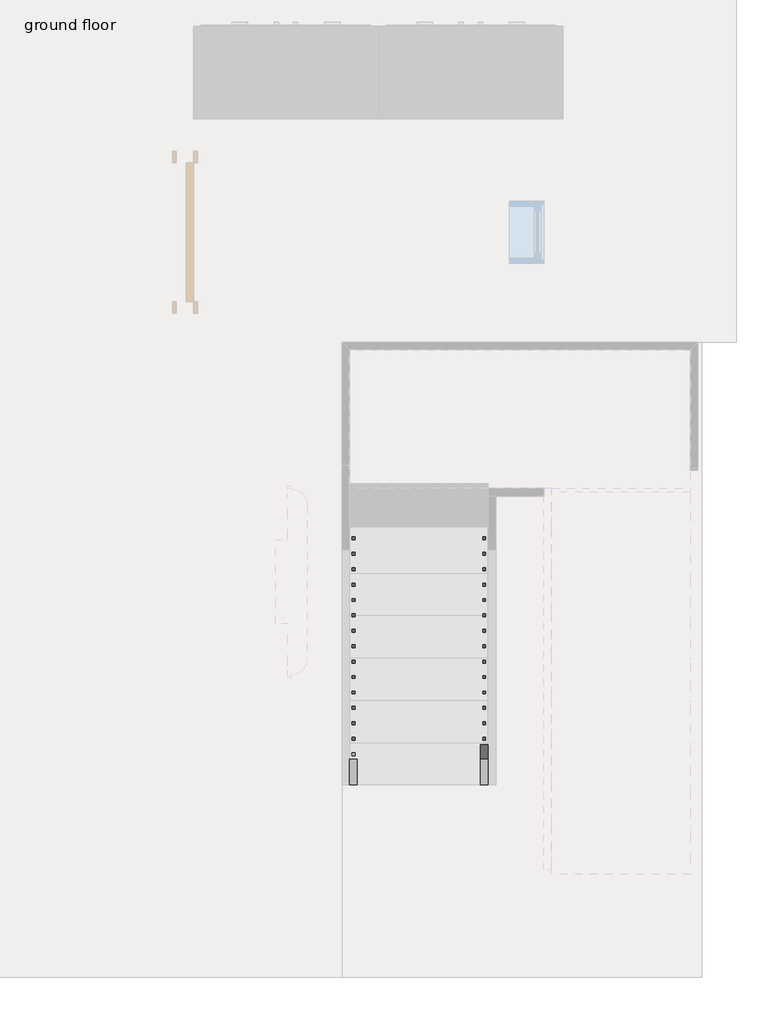
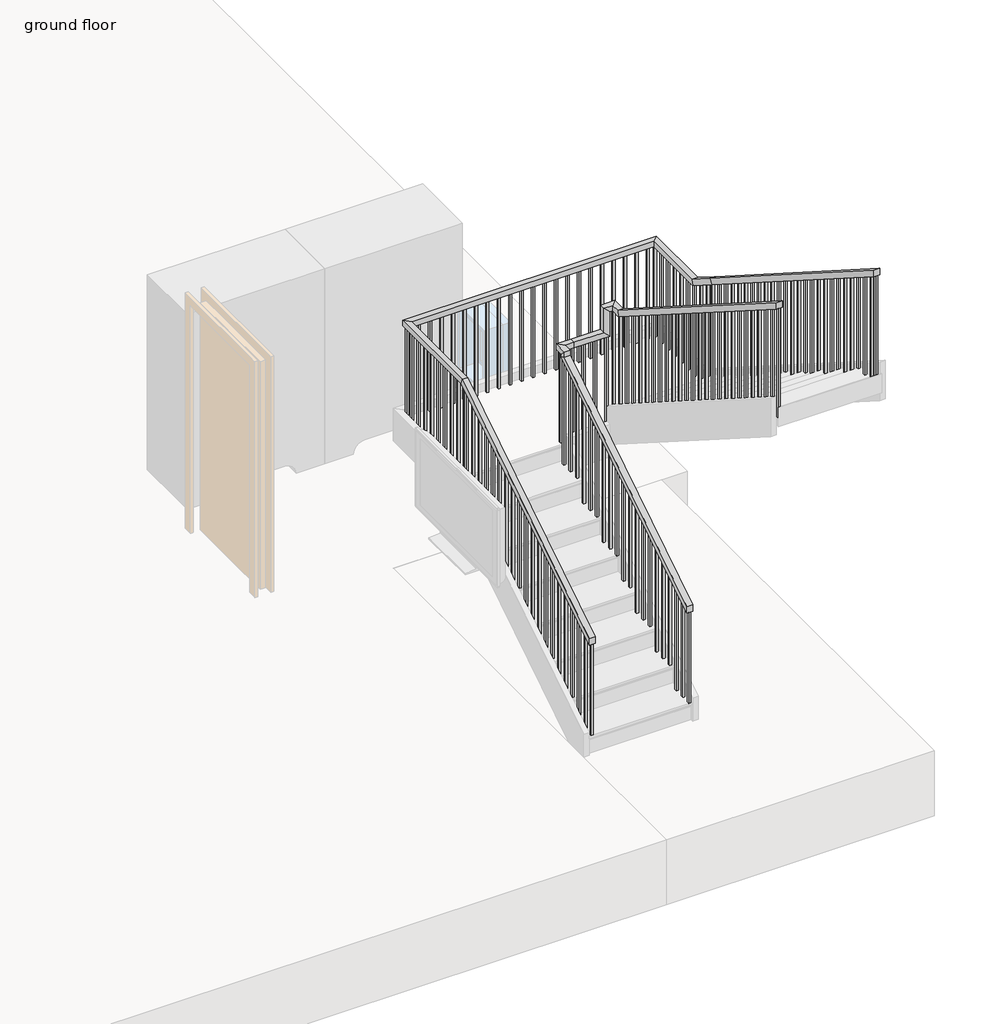
# One storey, part 2 of 3: 2 railings.
"""IFC4 building model written with IfcOpenShell, lengths in millimetres."""

from ifc_helpers import new_model, si_unit, frame, origin, place, context, project, spatial, polyline, outline, extrude, faceted_brep, element, save

model = new_model("IFC4")

# Units and contexts
model_context = context("Model", 3, world=origin())
ifc_project = project(units=[si_unit("LENGTHUNIT", "METRE", prefix="MILLI")], contexts=[model_context])

# Site, building, storey
site = spatial("IfcSite", under=ifc_project)
building = spatial("IfcBuilding", under=site)
storey = spatial("IfcBuildingStorey", under=building, Name="ground floor", Elevation=609.6)

# Railings
placement = place(None, origin())
element("IfcRailing", 1, ObjectType="Handrail - Rectangular", at=placement, inside=storey, context=model_context, shape_type="SolidModel", body=[
    faceted_brep([(995.5501403, 157.6257925, 1701.8), (995.5501403, 157.6257925, 1641.586276), (1046.3501403, 157.6257925, 1641.586276), (1046.3501403, 157.6257925, 1701.8), (995.5501403, 2037.2257925, 2897.9090909), (995.5501403, 2088.0257925, 2870.0226396), (1046.3501403, 2088.0257925, 2870.0226396), (1046.3501403, 2037.2257925, 2897.9090909), (995.5501403, 2037.2257925, 2946.4), (995.5501403, 2088.0257925, 2895.6), (1046.3501403, 2088.0257925, 2895.6), (1046.3501403, 2037.2257925, 2946.4), (995.5501403, 2164.2257925, 2946.4), (995.5501403, 2164.2257925, 2895.6), (1046.3501403, 2113.4257925, 2895.6), (1046.3501403, 2113.4257925, 2946.4), (1122.5501403, 2164.2257925, 2946.4), (1122.5501403, 2164.2257925, 2895.6), (1122.5501403, 2113.4257925, 2895.6), (1122.5501403, 2113.4257925, 2946.4), (1389.2501403, 2164.2257925, 2946.4), (1440.0501403, 2164.2257925, 2895.6), (1440.0501403, 2113.4257925, 2895.6), (1389.2501403, 2113.4257925, 2946.4), (1389.2501403, 2164.2257925, 3172.6909091), (1440.0501403, 2164.2257925, 3121.8909091), (1440.0501403, 2113.4257925, 3121.8909091), (1389.2501403, 2113.4257925, 3172.6909091), (1516.2501403, 2164.2257925, 3172.6909091), (1516.2501403, 2164.2257925, 3121.8909091), (1465.4501403, 2113.4257925, 3121.8909091), (1465.4501403, 2113.4257925, 3172.6909091), (1516.2501403, 2037.2257925, 3172.6909091), (1516.2501403, 2022.4327976, 3121.8909091), (1465.4501403, 2022.4327976, 3121.8909091), (1465.4501403, 2037.2257925, 3172.6909091), (1516.2501403, -401.1742075, 4724.4), (1465.4501403, -401.1742075, 4724.4), (1465.4501403, -401.1742075, 4664.186276), (1516.2501403, -401.1742075, 4664.186276)], [[[0, 1, 2, 3]], [[1, 0, 4, 5]], [[2, 1, 5, 6]], [[3, 2, 6, 7]], [[0, 3, 7, 4]], [[5, 4, 8, 9]], [[6, 5, 9, 10]], [[7, 6, 10, 11]], [[4, 7, 11, 8]], [[9, 8, 12, 13]], [[10, 9, 13, 14]], [[11, 10, 14, 15]], [[8, 11, 15, 12]], [[13, 12, 16, 17]], [[14, 13, 17, 18]], [[15, 14, 18, 19]], [[12, 15, 19, 16]], [[17, 16, 20, 21]], [[18, 17, 21, 22]], [[19, 18, 22, 23]], [[16, 19, 23, 20]], [[21, 20, 24, 25]], [[22, 21, 25, 26]], [[23, 22, 26, 27]], [[20, 23, 27, 24]], [[25, 24, 28, 29]], [[26, 25, 29, 30]], [[27, 26, 30, 31]], [[24, 27, 31, 28]], [[29, 28, 32, 33]], [[30, 29, 33, 34]], [[31, 30, 34, 35]], [[28, 31, 35, 32]], [[36, 37, 38, 39]], [[33, 32, 36, 39]], [[34, 33, 39, 38]], [[35, 34, 38, 37]], [[32, 35, 37, 36]]]),
    extrude(outline(polyline([(-309.0992075, 4605.5930941), (-290.0492075, 4593.4703669), (-290.0492075, 3632.2), (-309.0992075, 3632.2), (-309.0992075, 4605.5930941)])), frame((1481.3251403, 0.0, 0.0), z_axis=(1.0, 0.0, 0.0), x_axis=(0.0, 1.0, 0.0)), (0.0, 0.0, 1.0), 19.05),
    extrude(outline(polyline([(-207.4992075, 4540.9385487), (-188.4492075, 4528.8158214), (-188.4492075, 3632.2), (-207.4992075, 3632.2), (-207.4992075, 4540.9385487)])), frame((1481.3251403, 0.0, 0.0), z_axis=(1.0, 0.0, 0.0), x_axis=(0.0, 1.0, 0.0)), (0.0, 0.0, 1.0), 19.05),
    extrude(outline(polyline([(-105.8992075, 4476.2840032), (-86.8492075, 4464.161276), (-86.8492075, 3454.4), (-105.8992075, 3454.4), (-105.8992075, 4476.2840032)])), frame((1481.3251403, 0.0, 0.0), z_axis=(1.0, 0.0, 0.0), x_axis=(0.0, 1.0, 0.0)), (0.0, 0.0, 1.0), 19.05),
    extrude(outline(polyline([(-4.2992075, 4411.6294578), (14.7507925, 4399.5067305), (14.7507925, 3454.4), (-4.2992075, 3454.4), (-4.2992075, 4411.6294578)])), frame((1481.3251403, 0.0, 0.0), z_axis=(1.0, 0.0, 0.0), x_axis=(0.0, 1.0, 0.0)), (0.0, 0.0, 1.0), 19.05),
    extrude(outline(polyline([(97.3007925, 4346.9749123), (116.3507925, 4334.8521851), (116.3507925, 3454.4), (97.3007925, 3454.4), (97.3007925, 4346.9749123)])), frame((1481.3251403, 0.0, 0.0), z_axis=(1.0, 0.0, 0.0), x_axis=(0.0, 1.0, 0.0)), (0.0, 0.0, 1.0), 19.05),
    extrude(outline(polyline([(198.9007925, 4282.3203669), (217.9507925, 4270.1976396), (217.9507925, 3276.6), (198.9007925, 3276.6), (198.9007925, 4282.3203669)])), frame((1481.3251403, 0.0, 0.0), z_axis=(1.0, 0.0, 0.0), x_axis=(0.0, 1.0, 0.0)), (0.0, 0.0, 1.0), 19.05),
    extrude(outline(polyline([(300.5007925, 4217.6658214), (319.5507925, 4205.5430941), (319.5507925, 3276.6), (300.5007925, 3276.6), (300.5007925, 4217.6658214)])), frame((1481.3251403, 0.0, 0.0), z_axis=(1.0, 0.0, 0.0), x_axis=(0.0, 1.0, 0.0)), (0.0, 0.0, 1.0), 19.05),
    extrude(outline(polyline([(402.1007925, 4153.011276), (421.1507925, 4140.8885487), (421.1507925, 3276.6), (402.1007925, 3276.6), (402.1007925, 4153.011276)])), frame((1481.3251403, 0.0, 0.0), z_axis=(1.0, 0.0, 0.0), x_axis=(0.0, 1.0, 0.0)), (0.0, 0.0, 1.0), 19.05),
    extrude(outline(polyline([(503.7007925, 4088.3567305), (522.7507925, 4076.2340032), (522.7507925, 3098.8), (503.7007925, 3098.8), (503.7007925, 4088.3567305)])), frame((1481.3251403, 0.0, 0.0), z_axis=(1.0, 0.0, 0.0), x_axis=(0.0, 1.0, 0.0)), (0.0, 0.0, 1.0), 19.05),
    extrude(outline(polyline([(605.3007925, 4023.7021851), (624.3507925, 4011.5794578), (624.3507925, 3098.8), (605.3007925, 3098.8), (605.3007925, 4023.7021851)])), frame((1481.3251403, 0.0, 0.0), z_axis=(1.0, 0.0, 0.0), x_axis=(0.0, 1.0, 0.0)), (0.0, 0.0, 1.0), 19.05),
    extrude(outline(polyline([(706.9007925, 3959.0476396), (725.9507925, 3946.9249123), (725.9507925, 3098.8), (706.9007925, 3098.8), (706.9007925, 3959.0476396)])), frame((1481.3251403, 0.0, 0.0), z_axis=(1.0, 0.0, 0.0), x_axis=(0.0, 1.0, 0.0)), (0.0, 0.0, 1.0), 19.05),
    extrude(outline(polyline([(808.5007925, 3894.3930941), (827.5507925, 3882.2703669), (827.5507925, 2921.0), (808.5007925, 2921.0), (808.5007925, 3894.3930941)])), frame((1481.3251403, 0.0, 0.0), z_axis=(1.0, 0.0, 0.0), x_axis=(0.0, 1.0, 0.0)), (0.0, 0.0, 1.0), 19.05),
    extrude(outline(polyline([(910.1007925, 3829.7385487), (929.1507925, 3817.6158214), (929.1507925, 2921.0), (910.1007925, 2921.0), (910.1007925, 3829.7385487)])), frame((1481.3251403, 0.0, 0.0), z_axis=(1.0, 0.0, 0.0), x_axis=(0.0, 1.0, 0.0)), (0.0, 0.0, 1.0), 19.05),
    extrude(outline(polyline([(1011.7007925, 3765.0840032), (1030.7507925, 3752.961276), (1030.7507925, 2743.2), (1011.7007925, 2743.2), (1011.7007925, 3765.0840032)])), frame((1481.3251403, 0.0, 0.0), z_axis=(1.0, 0.0, 0.0), x_axis=(0.0, 1.0, 0.0)), (0.0, 0.0, 1.0), 19.05),
    extrude(outline(polyline([(1113.3007925, 3700.4294578), (1132.3507925, 3688.3067305), (1132.3507925, 2743.2), (1113.3007925, 2743.2), (1113.3007925, 3700.4294578)])), frame((1481.3251403, 0.0, 0.0), z_axis=(1.0, 0.0, 0.0), x_axis=(0.0, 1.0, 0.0)), (0.0, 0.0, 1.0), 19.05),
    extrude(outline(polyline([(1214.9007925, 3635.7749123), (1233.9507925, 3623.6521851), (1233.9507925, 2743.2), (1214.9007925, 2743.2), (1214.9007925, 3635.7749123)])), frame((1481.3251403, 0.0, 0.0), z_axis=(1.0, 0.0, 0.0), x_axis=(0.0, 1.0, 0.0)), (0.0, 0.0, 1.0), 19.05),
    extrude(outline(polyline([(1316.5007925, 3571.1203669), (1335.5507925, 3558.9976396), (1335.5507925, 2565.4), (1316.5007925, 2565.4), (1316.5007925, 3571.1203669)])), frame((1481.3251403, 0.0, 0.0), z_axis=(1.0, 0.0, 0.0), x_axis=(0.0, 1.0, 0.0)), (0.0, 0.0, 1.0), 19.05),
    extrude(outline(polyline([(1418.1007925, 3506.4658214), (1437.1507925, 3494.3430941), (1437.1507925, 2565.4), (1418.1007925, 2565.4), (1418.1007925, 3506.4658214)])), frame((1481.3251403, 0.0, 0.0), z_axis=(1.0, 0.0, 0.0), x_axis=(0.0, 1.0, 0.0)), (0.0, 0.0, 1.0), 19.05),
    extrude(outline(polyline([(1519.7007925, 3441.811276), (1538.7507925, 3429.6885487), (1538.7507925, 2565.4), (1519.7007925, 2565.4), (1519.7007925, 3441.811276)])), frame((1481.3251403, 0.0, 0.0), z_axis=(1.0, 0.0, 0.0), x_axis=(0.0, 1.0, 0.0)), (0.0, 0.0, 1.0), 19.05),
    extrude(outline(polyline([(1621.3007925, 3377.1567305), (1640.3507925, 3365.0340032), (1640.3507925, 2387.6), (1621.3007925, 2387.6), (1621.3007925, 3377.1567305)])), frame((1481.3251403, 0.0, 0.0), z_axis=(1.0, 0.0, 0.0), x_axis=(0.0, 1.0, 0.0)), (0.0, 0.0, 1.0), 19.05),
    extrude(outline(polyline([(1722.9007925, 3312.5021851), (1741.9507925, 3300.3794578), (1741.9507925, 2387.6), (1722.9007925, 2387.6), (1722.9007925, 3312.5021851)])), frame((1481.3251403, 0.0, 0.0), z_axis=(1.0, 0.0, 0.0), x_axis=(0.0, 1.0, 0.0)), (0.0, 0.0, 1.0), 19.05),
    extrude(outline(polyline([(1824.5007925, 3247.8476396), (1843.5507925, 3235.7249123), (1843.5507925, 2387.6), (1824.5007925, 2387.6), (1824.5007925, 3247.8476396)])), frame((1481.3251403, 0.0, 0.0), z_axis=(1.0, 0.0, 0.0), x_axis=(0.0, 1.0, 0.0)), (0.0, 0.0, 1.0), 19.05),
    extrude(outline(polyline([(1926.1007925, 3183.1930941), (1945.1507925, 3171.0703669), (1945.1507925, 2209.8), (1926.1007925, 2209.8), (1926.1007925, 3183.1930941)])), frame((1481.3251403, 0.0, 0.0), z_axis=(1.0, 0.0, 0.0), x_axis=(0.0, 1.0, 0.0)), (0.0, 0.0, 1.0), 19.05),
    extrude(outline(polyline([(2027.7007925, 3118.5385487), (2046.7507925, 3106.4158214), (2046.7507925, 2209.8), (2027.7007925, 2209.8), (2027.7007925, 3118.5385487)])), frame((1481.3251403, 0.0, 0.0), z_axis=(1.0, 0.0, 0.0), x_axis=(0.0, 1.0, 0.0)), (0.0, 0.0, 1.0), 19.05),
    extrude(outline(polyline([(1417.8251403, 2129.3007925), (1417.8251403, 2148.3507925), (1436.8751403, 2148.3507925), (1436.8751403, 2129.3007925), (1417.8251403, 2129.3007925)])), frame((0.0, 0.0, 2032.0), z_axis=(0.0, 0.0, 1.0), x_axis=(1.0, 0.0, 0.0)), (0.0, 0.0, 1.0), 1089.8909091),
    extrude(outline(polyline([(1316.2251403, 2129.3007925), (1316.2251403, 2148.3507925), (1335.2751403, 2148.3507925), (1335.2751403, 2129.3007925), (1316.2251403, 2129.3007925)])), frame((0.0, 0.0, 2032.0), z_axis=(0.0, 0.0, 1.0), x_axis=(1.0, 0.0, 0.0)), (0.0, 0.0, 1.0), 863.6),
    extrude(outline(polyline([(1214.6251403, 2129.3007925), (1214.6251403, 2148.3507925), (1233.6751403, 2148.3507925), (1233.6751403, 2129.3007925), (1214.6251403, 2129.3007925)])), frame((0.0, 0.0, 2032.0), z_axis=(0.0, 0.0, 1.0), x_axis=(1.0, 0.0, 0.0)), (0.0, 0.0, 1.0), 863.6),
    extrude(outline(polyline([(1113.0251403, 2129.3007925), (1113.0251403, 2148.3507925), (1132.0751403, 2148.3507925), (1132.0751403, 2129.3007925), (1113.0251403, 2129.3007925)])), frame((0.0, 0.0, 2032.0), z_axis=(0.0, 0.0, 1.0), x_axis=(1.0, 0.0, 0.0)), (0.0, 0.0, 1.0), 863.6),
    extrude(outline(polyline([(1030.4751403, 2078.5007925), (1011.4251403, 2078.5007925), (1011.4251403, 2097.5507925), (1030.4751403, 2097.5507925), (1030.4751403, 2078.5007925)])), frame((0.0, 0.0, 1854.2), z_axis=(0.0, 0.0, 1.0), x_axis=(1.0, 0.0, 0.0)), (0.0, 0.0, 1.0), 1041.4),
    extrude(outline(polyline([(1976.9007925, 2799.3067305), (1995.9507925, 2811.4294578), (1995.9507925, 1854.2), (1976.9007925, 1854.2), (1976.9007925, 2799.3067305)])), frame((1011.4251403, 0.0, 0.0), z_axis=(1.0, 0.0, 0.0), x_axis=(0.0, 1.0, 0.0)), (0.0, 0.0, 1.0), 19.05),
    extrude(outline(polyline([(1875.3007925, 2734.6521851), (1894.3507925, 2746.7749123), (1894.3507925, 1854.2), (1875.3007925, 1854.2), (1875.3007925, 2734.6521851)])), frame((1011.4251403, 0.0, 0.0), z_axis=(1.0, 0.0, 0.0), x_axis=(0.0, 1.0, 0.0)), (0.0, 0.0, 1.0), 19.05),
    extrude(outline(polyline([(1773.7007925, 2669.9976396), (1792.7507925, 2682.1203669), (1792.7507925, 1676.4), (1773.7007925, 1676.4), (1773.7007925, 2669.9976396)])), frame((1011.4251403, 0.0, 0.0), z_axis=(1.0, 0.0, 0.0), x_axis=(0.0, 1.0, 0.0)), (0.0, 0.0, 1.0), 19.05),
    extrude(outline(polyline([(1672.1007925, 2605.3430941), (1691.1507925, 2617.4658214), (1691.1507925, 1676.4), (1672.1007925, 1676.4), (1672.1007925, 2605.3430941)])), frame((1011.4251403, 0.0, 0.0), z_axis=(1.0, 0.0, 0.0), x_axis=(0.0, 1.0, 0.0)), (0.0, 0.0, 1.0), 19.05),
    extrude(outline(polyline([(1570.5007925, 2540.6885487), (1589.5507925, 2552.811276), (1589.5507925, 1676.4), (1570.5007925, 1676.4), (1570.5007925, 2540.6885487)])), frame((1011.4251403, 0.0, 0.0), z_axis=(1.0, 0.0, 0.0), x_axis=(0.0, 1.0, 0.0)), (0.0, 0.0, 1.0), 19.05),
    extrude(outline(polyline([(1468.9007925, 2476.0340032), (1487.9507925, 2488.1567305), (1487.9507925, 1498.6), (1468.9007925, 1498.6), (1468.9007925, 2476.0340032)])), frame((1011.4251403, 0.0, 0.0), z_axis=(1.0, 0.0, 0.0), x_axis=(0.0, 1.0, 0.0)), (0.0, 0.0, 1.0), 19.05),
    extrude(outline(polyline([(1367.3007925, 2411.3794578), (1386.3507925, 2423.5021851), (1386.3507925, 1498.6), (1367.3007925, 1498.6), (1367.3007925, 2411.3794578)])), frame((1011.4251403, 0.0, 0.0), z_axis=(1.0, 0.0, 0.0), x_axis=(0.0, 1.0, 0.0)), (0.0, 0.0, 1.0), 19.05),
    extrude(outline(polyline([(1265.7007925, 2346.7249123), (1284.7507925, 2358.8476396), (1284.7507925, 1498.6), (1265.7007925, 1498.6), (1265.7007925, 2346.7249123)])), frame((1011.4251403, 0.0, 0.0), z_axis=(1.0, 0.0, 0.0), x_axis=(0.0, 1.0, 0.0)), (0.0, 0.0, 1.0), 19.05),
    extrude(outline(polyline([(1164.1007925, 2282.0703669), (1183.1507925, 2294.1930941), (1183.1507925, 1320.8), (1164.1007925, 1320.8), (1164.1007925, 2282.0703669)])), frame((1011.4251403, 0.0, 0.0), z_axis=(1.0, 0.0, 0.0), x_axis=(0.0, 1.0, 0.0)), (0.0, 0.0, 1.0), 19.05),
    extrude(outline(polyline([(1062.5007925, 2217.4158214), (1081.5507925, 2229.5385487), (1081.5507925, 1320.8), (1062.5007925, 1320.8), (1062.5007925, 2217.4158214)])), frame((1011.4251403, 0.0, 0.0), z_axis=(1.0, 0.0, 0.0), x_axis=(0.0, 1.0, 0.0)), (0.0, 0.0, 1.0), 19.05),
    extrude(outline(polyline([(960.9007925, 2152.761276), (979.9507925, 2164.8840032), (979.9507925, 1143.0), (960.9007925, 1143.0), (960.9007925, 2152.761276)])), frame((1011.4251403, 0.0, 0.0), z_axis=(1.0, 0.0, 0.0), x_axis=(0.0, 1.0, 0.0)), (0.0, 0.0, 1.0), 19.05),
    extrude(outline(polyline([(859.3007925, 2088.1067305), (878.3507925, 2100.2294578), (878.3507925, 1143.0), (859.3007925, 1143.0), (859.3007925, 2088.1067305)])), frame((1011.4251403, 0.0, 0.0), z_axis=(1.0, 0.0, 0.0), x_axis=(0.0, 1.0, 0.0)), (0.0, 0.0, 1.0), 19.05),
    extrude(outline(polyline([(757.7007925, 2023.4521851), (776.7507925, 2035.5749123), (776.7507925, 1143.0), (757.7007925, 1143.0), (757.7007925, 2023.4521851)])), frame((1011.4251403, 0.0, 0.0), z_axis=(1.0, 0.0, 0.0), x_axis=(0.0, 1.0, 0.0)), (0.0, 0.0, 1.0), 19.05),
    extrude(outline(polyline([(656.1007925, 1958.7976396), (675.1507925, 1970.9203669), (675.1507925, 965.2), (656.1007925, 965.2), (656.1007925, 1958.7976396)])), frame((1011.4251403, 0.0, 0.0), z_axis=(1.0, 0.0, 0.0), x_axis=(0.0, 1.0, 0.0)), (0.0, 0.0, 1.0), 19.05),
    extrude(outline(polyline([(554.5007925, 1894.1430941), (573.5507925, 1906.2658214), (573.5507925, 965.2), (554.5007925, 965.2), (554.5007925, 1894.1430941)])), frame((1011.4251403, 0.0, 0.0), z_axis=(1.0, 0.0, 0.0), x_axis=(0.0, 1.0, 0.0)), (0.0, 0.0, 1.0), 19.05),
    extrude(outline(polyline([(452.9007925, 1829.4885487), (471.9507925, 1841.611276), (471.9507925, 965.2), (452.9007925, 965.2), (452.9007925, 1829.4885487)])), frame((1011.4251403, 0.0, 0.0), z_axis=(1.0, 0.0, 0.0), x_axis=(0.0, 1.0, 0.0)), (0.0, 0.0, 1.0), 19.05),
    extrude(outline(polyline([(351.3007925, 1764.8340032), (370.3507925, 1776.9567305), (370.3507925, 787.4), (351.3007925, 787.4), (351.3007925, 1764.8340032)])), frame((1011.4251403, 0.0, 0.0), z_axis=(1.0, 0.0, 0.0), x_axis=(0.0, 1.0, 0.0)), (0.0, 0.0, 1.0), 19.05),
    extrude(outline(polyline([(249.7007925, 1700.1794578), (268.7507925, 1712.3021851), (268.7507925, 787.4), (249.7007925, 787.4), (249.7007925, 1700.1794578)])), frame((1011.4251403, 0.0, 0.0), z_axis=(1.0, 0.0, 0.0), x_axis=(0.0, 1.0, 0.0)), (0.0, 0.0, 1.0), 19.05),
    extrude(outline(polyline([(1481.3251403, 2129.3007925), (1481.3251403, 2148.3507925), (1500.3751403, 2148.3507925), (1500.3751403, 2129.3007925), (1481.3251403, 2129.3007925)])), frame((0.0, 0.0, 2032.0), z_axis=(0.0, 0.0, 1.0), x_axis=(1.0, 0.0, 0.0)), (0.0, 0.0, 1.0), 1089.8909091),
    extrude(outline(polyline([(1030.4751403, 2129.3007925), (1011.4251403, 2129.3007925), (1011.4251403, 2148.3507925), (1030.4751403, 2148.3507925), (1030.4751403, 2129.3007925)])), frame((0.0, 0.0, 2032.0), z_axis=(0.0, 0.0, 1.0), x_axis=(1.0, 0.0, 0.0)), (0.0, 0.0, 1.0), 863.6),
    extrude(outline(polyline([(-401.1742075, 4664.186276), (-382.1242075, 4652.0635487), (-382.1242075, 3632.2), (-401.1742075, 3632.2), (-401.1742075, 4664.186276)])), frame((1481.3251403, 0.0, 0.0), z_axis=(1.0, 0.0, 0.0), x_axis=(0.0, 1.0, 0.0)), (0.0, 0.0, 1.0), 19.05),
    extrude(outline(polyline([(157.6257925, 1641.586276), (176.6757925, 1653.7090032), (176.6757925, 787.4), (157.6257925, 787.4), (157.6257925, 1641.586276)])), frame((1011.4251403, 0.0, 0.0), z_axis=(1.0, 0.0, 0.0), x_axis=(0.0, 1.0, 0.0)), (0.0, 0.0, 1.0), 19.05),
])
element("IfcRailing", 2, ObjectType="Handrail - Rectangular", at=placement, inside=storey, context=model_context, shape_type="SolidModel", body=[
    faceted_brep([(131.9501403, 157.6257925, 1701.8), (131.9501403, 157.6257925, 1641.586276), (182.7501403, 157.6257925, 1641.586276), (182.7501403, 157.6257925, 1701.8), (131.9501403, 2113.4257925, 2946.4), (131.9501403, 2128.2187874, 2895.6), (182.7501403, 2128.2187874, 2895.6), (182.7501403, 2113.4257925, 2946.4), (131.9501403, 3027.8257925, 2946.4), (131.9501403, 3027.8257925, 2895.6), (182.7501403, 2977.0257925, 2895.6), (182.7501403, 2977.0257925, 2946.4), (2379.8501403, 3027.8257925, 2946.4), (2379.8501403, 3027.8257925, 2895.6), (2329.0501403, 2977.0257925, 2895.6), (2329.0501403, 2977.0257925, 2946.4), (2379.8501403, 2392.8257925, 2946.4), (2379.8501403, 2378.0327976, 2895.6), (2329.0501403, 2378.0327976, 2895.6), (2329.0501403, 2392.8257925, 2946.4), (2379.8501403, 2113.4257925, 3124.2), (2379.8501403, 2086.1525175, 3081.3419964), (2329.0501403, 2086.1525175, 3081.3419964), (2329.0501403, 2113.4257925, 3124.2), (2379.8501403, -401.1742075, 4724.4), (2329.0501403, -401.1742075, 4724.4), (2329.0501403, -401.1742075, 4664.186276), (2379.8501403, -401.1742075, 4664.186276)], [[[0, 1, 2, 3]], [[1, 0, 4, 5]], [[2, 1, 5, 6]], [[3, 2, 6, 7]], [[0, 3, 7, 4]], [[5, 4, 8, 9]], [[6, 5, 9, 10]], [[7, 6, 10, 11]], [[4, 7, 11, 8]], [[9, 8, 12, 13]], [[10, 9, 13, 14]], [[11, 10, 14, 15]], [[8, 11, 15, 12]], [[13, 12, 16, 17]], [[14, 13, 17, 18]], [[15, 14, 18, 19]], [[12, 15, 19, 16]], [[17, 16, 20, 21]], [[18, 17, 21, 22]], [[19, 18, 22, 23]], [[16, 19, 23, 20]], [[24, 25, 26, 27]], [[21, 20, 24, 27]], [[22, 21, 27, 26]], [[23, 22, 26, 25]], [[20, 23, 25, 24]]]),
    extrude(outline(polyline([(-315.4492075, 4609.6340032), (-315.4492075, 3632.2), (-334.4992075, 3632.2), (-334.4992075, 4621.7567305), (-315.4492075, 4609.6340032)])), frame((2344.9251403, 0.0, 0.0), z_axis=(1.0, 0.0, 0.0), x_axis=(0.0, 1.0, 0.0)), (0.0, 0.0, 1.0), 19.05),
    extrude(outline(polyline([(-213.8492075, 4544.9794578), (-213.8492075, 3632.2), (-232.8992075, 3632.2), (-232.8992075, 4557.1021851), (-213.8492075, 4544.9794578)])), frame((2344.9251403, 0.0, 0.0), z_axis=(1.0, 0.0, 0.0), x_axis=(0.0, 1.0, 0.0)), (0.0, 0.0, 1.0), 19.05),
    extrude(outline(polyline([(-112.2492075, 4480.3249123), (-112.2492075, 3632.2), (-131.2992075, 3632.2), (-131.2992075, 4492.4476396), (-112.2492075, 4480.3249123)])), frame((2344.9251403, 0.0, 0.0), z_axis=(1.0, 0.0, 0.0), x_axis=(0.0, 1.0, 0.0)), (0.0, 0.0, 1.0), 19.05),
    extrude(outline(polyline([(-10.6492075, 4415.6703669), (-10.6492075, 3454.4), (-29.6992075, 3454.4), (-29.6992075, 4427.7930941), (-10.6492075, 4415.6703669)])), frame((2344.9251403, 0.0, 0.0), z_axis=(1.0, 0.0, 0.0), x_axis=(0.0, 1.0, 0.0)), (0.0, 0.0, 1.0), 19.05),
    extrude(outline(polyline([(90.9507925, 4351.0158214), (90.9507925, 3454.4), (71.9007925, 3454.4), (71.9007925, 4363.1385487), (90.9507925, 4351.0158214)])), frame((2344.9251403, 0.0, 0.0), z_axis=(1.0, 0.0, 0.0), x_axis=(0.0, 1.0, 0.0)), (0.0, 0.0, 1.0), 19.05),
    extrude(outline(polyline([(192.5507925, 4286.361276), (192.5507925, 3276.6), (173.5007925, 3276.6), (173.5007925, 4298.4840032), (192.5507925, 4286.361276)])), frame((2344.9251403, 0.0, 0.0), z_axis=(1.0, 0.0, 0.0), x_axis=(0.0, 1.0, 0.0)), (0.0, 0.0, 1.0), 19.05),
    extrude(outline(polyline([(294.1507925, 4221.7067305), (294.1507925, 3276.6), (275.1007925, 3276.6), (275.1007925, 4233.8294578), (294.1507925, 4221.7067305)])), frame((2344.9251403, 0.0, 0.0), z_axis=(1.0, 0.0, 0.0), x_axis=(0.0, 1.0, 0.0)), (0.0, 0.0, 1.0), 19.05),
    extrude(outline(polyline([(395.7507925, 4157.0521851), (395.7507925, 3276.6), (376.7007925, 3276.6), (376.7007925, 4169.1749123), (395.7507925, 4157.0521851)])), frame((2344.9251403, 0.0, 0.0), z_axis=(1.0, 0.0, 0.0), x_axis=(0.0, 1.0, 0.0)), (0.0, 0.0, 1.0), 19.05),
    extrude(outline(polyline([(497.3507925, 4092.3976396), (497.3507925, 3098.8), (478.3007925, 3098.8), (478.3007925, 4104.5203669), (497.3507925, 4092.3976396)])), frame((2344.9251403, 0.0, 0.0), z_axis=(1.0, 0.0, 0.0), x_axis=(0.0, 1.0, 0.0)), (0.0, 0.0, 1.0), 19.05),
    extrude(outline(polyline([(598.9507925, 4027.7430941), (598.9507925, 3098.8), (579.9007925, 3098.8), (579.9007925, 4039.8658214), (598.9507925, 4027.7430941)])), frame((2344.9251403, 0.0, 0.0), z_axis=(1.0, 0.0, 0.0), x_axis=(0.0, 1.0, 0.0)), (0.0, 0.0, 1.0), 19.05),
    extrude(outline(polyline([(700.5507925, 3963.0885487), (700.5507925, 3098.8), (681.5007925, 3098.8), (681.5007925, 3975.211276), (700.5507925, 3963.0885487)])), frame((2344.9251403, 0.0, 0.0), z_axis=(1.0, 0.0, 0.0), x_axis=(0.0, 1.0, 0.0)), (0.0, 0.0, 1.0), 19.05),
    extrude(outline(polyline([(802.1507925, 3898.4340032), (802.1507925, 2921.0), (783.1007925, 2921.0), (783.1007925, 3910.5567305), (802.1507925, 3898.4340032)])), frame((2344.9251403, 0.0, 0.0), z_axis=(1.0, 0.0, 0.0), x_axis=(0.0, 1.0, 0.0)), (0.0, 0.0, 1.0), 19.05),
    extrude(outline(polyline([(903.7507925, 3833.7794578), (903.7507925, 2921.0), (884.7007925, 2921.0), (884.7007925, 3845.9021851), (903.7507925, 3833.7794578)])), frame((2344.9251403, 0.0, 0.0), z_axis=(1.0, 0.0, 0.0), x_axis=(0.0, 1.0, 0.0)), (0.0, 0.0, 1.0), 19.05),
    extrude(outline(polyline([(1005.3507925, 3769.1249123), (1005.3507925, 2921.0), (986.3007925, 2921.0), (986.3007925, 3781.2476396), (1005.3507925, 3769.1249123)])), frame((2344.9251403, 0.0, 0.0), z_axis=(1.0, 0.0, 0.0), x_axis=(0.0, 1.0, 0.0)), (0.0, 0.0, 1.0), 19.05),
    extrude(outline(polyline([(1106.9507925, 3704.4703669), (1106.9507925, 2743.2), (1087.9007925, 2743.2), (1087.9007925, 3716.5930941), (1106.9507925, 3704.4703669)])), frame((2344.9251403, 0.0, 0.0), z_axis=(1.0, 0.0, 0.0), x_axis=(0.0, 1.0, 0.0)), (0.0, 0.0, 1.0), 19.05),
    extrude(outline(polyline([(1208.5507925, 3639.8158214), (1208.5507925, 2743.2), (1189.5007925, 2743.2), (1189.5007925, 3651.9385487), (1208.5507925, 3639.8158214)])), frame((2344.9251403, 0.0, 0.0), z_axis=(1.0, 0.0, 0.0), x_axis=(0.0, 1.0, 0.0)), (0.0, 0.0, 1.0), 19.05),
    extrude(outline(polyline([(1310.1507925, 3575.161276), (1310.1507925, 2565.4), (1291.1007925, 2565.4), (1291.1007925, 3587.2840032), (1310.1507925, 3575.161276)])), frame((2344.9251403, 0.0, 0.0), z_axis=(1.0, 0.0, 0.0), x_axis=(0.0, 1.0, 0.0)), (0.0, 0.0, 1.0), 19.05),
    extrude(outline(polyline([(1411.7507925, 3510.5067305), (1411.7507925, 2565.4), (1392.7007925, 2565.4), (1392.7007925, 3522.6294578), (1411.7507925, 3510.5067305)])), frame((2344.9251403, 0.0, 0.0), z_axis=(1.0, 0.0, 0.0), x_axis=(0.0, 1.0, 0.0)), (0.0, 0.0, 1.0), 19.05),
    extrude(outline(polyline([(1513.3507925, 3445.8521851), (1513.3507925, 2565.4), (1494.3007925, 2565.4), (1494.3007925, 3457.9749123), (1513.3507925, 3445.8521851)])), frame((2344.9251403, 0.0, 0.0), z_axis=(1.0, 0.0, 0.0), x_axis=(0.0, 1.0, 0.0)), (0.0, 0.0, 1.0), 19.05),
    extrude(outline(polyline([(1614.9507925, 3381.1976396), (1614.9507925, 2387.6), (1595.9007925, 2387.6), (1595.9007925, 3393.3203669), (1614.9507925, 3381.1976396)])), frame((2344.9251403, 0.0, 0.0), z_axis=(1.0, 0.0, 0.0), x_axis=(0.0, 1.0, 0.0)), (0.0, 0.0, 1.0), 19.05),
    extrude(outline(polyline([(1716.5507925, 3316.5430941), (1716.5507925, 2387.6), (1697.5007925, 2387.6), (1697.5007925, 3328.6658214), (1716.5507925, 3316.5430941)])), frame((2344.9251403, 0.0, 0.0), z_axis=(1.0, 0.0, 0.0), x_axis=(0.0, 1.0, 0.0)), (0.0, 0.0, 1.0), 19.05),
    extrude(outline(polyline([(1818.1507925, 3251.8885487), (1818.1507925, 2387.6), (1799.1007925, 2387.6), (1799.1007925, 3264.011276), (1818.1507925, 3251.8885487)])), frame((2344.9251403, 0.0, 0.0), z_axis=(1.0, 0.0, 0.0), x_axis=(0.0, 1.0, 0.0)), (0.0, 0.0, 1.0), 19.05),
    extrude(outline(polyline([(1919.7507925, 3187.2340032), (1919.7507925, 2209.8), (1900.7007925, 2209.8), (1900.7007925, 3199.3567305), (1919.7507925, 3187.2340032)])), frame((2344.9251403, 0.0, 0.0), z_axis=(1.0, 0.0, 0.0), x_axis=(0.0, 1.0, 0.0)), (0.0, 0.0, 1.0), 19.05),
    extrude(outline(polyline([(2021.3507925, 3122.5794578), (2021.3507925, 2209.8), (2002.3007925, 2209.8), (2002.3007925, 3134.7021851), (2021.3507925, 3122.5794578)])), frame((2344.9251403, 0.0, 0.0), z_axis=(1.0, 0.0, 0.0), x_axis=(0.0, 1.0, 0.0)), (0.0, 0.0, 1.0), 19.05),
    extrude(outline(polyline([(2199.1507925, 3009.4340032), (2199.1507925, 2032.0), (2180.1007925, 2032.0), (2180.1007925, 3021.5567305), (2199.1507925, 3009.4340032)])), frame((2344.9251403, 0.0, 0.0), z_axis=(1.0, 0.0, 0.0), x_axis=(0.0, 1.0, 0.0)), (0.0, 0.0, 1.0), 19.05),
    extrude(outline(polyline([(2300.7507925, 2944.7794578), (2300.7507925, 2032.0), (2281.7007925, 2032.0), (2281.7007925, 2956.9021851), (2300.7507925, 2944.7794578)])), frame((2344.9251403, 0.0, 0.0), z_axis=(1.0, 0.0, 0.0), x_axis=(0.0, 1.0, 0.0)), (0.0, 0.0, 1.0), 19.05),
    extrude(outline(polyline([(2363.9751403, 2402.3507925), (2363.9751403, 2383.3007925), (2344.9251403, 2383.3007925), (2344.9251403, 2402.3507925), (2363.9751403, 2402.3507925)])), frame((0.0, 0.0, 2032.0), z_axis=(0.0, 0.0, 1.0), x_axis=(1.0, 0.0, 0.0)), (0.0, 0.0, 1.0), 863.6),
    extrude(outline(polyline([(2363.9751403, 2503.9507925), (2363.9751403, 2484.9007925), (2344.9251403, 2484.9007925), (2344.9251403, 2503.9507925), (2363.9751403, 2503.9507925)])), frame((0.0, 0.0, 2032.0), z_axis=(0.0, 0.0, 1.0), x_axis=(1.0, 0.0, 0.0)), (0.0, 0.0, 1.0), 863.6),
    extrude(outline(polyline([(2363.9751403, 2605.5507925), (2363.9751403, 2586.5007925), (2344.9251403, 2586.5007925), (2344.9251403, 2605.5507925), (2363.9751403, 2605.5507925)])), frame((0.0, 0.0, 2032.0), z_axis=(0.0, 0.0, 1.0), x_axis=(1.0, 0.0, 0.0)), (0.0, 0.0, 1.0), 863.6),
    extrude(outline(polyline([(2363.9751403, 2707.1507925), (2363.9751403, 2688.1007925), (2344.9251403, 2688.1007925), (2344.9251403, 2707.1507925), (2363.9751403, 2707.1507925)])), frame((0.0, 0.0, 2032.0), z_axis=(0.0, 0.0, 1.0), x_axis=(1.0, 0.0, 0.0)), (0.0, 0.0, 1.0), 863.6),
    extrude(outline(polyline([(2363.9751403, 2808.7507925), (2363.9751403, 2789.7007925), (2344.9251403, 2789.7007925), (2344.9251403, 2808.7507925), (2363.9751403, 2808.7507925)])), frame((0.0, 0.0, 2032.0), z_axis=(0.0, 0.0, 1.0), x_axis=(1.0, 0.0, 0.0)), (0.0, 0.0, 1.0), 863.6),
    extrude(outline(polyline([(2363.9751403, 2910.3507925), (2363.9751403, 2891.3007925), (2344.9251403, 2891.3007925), (2344.9251403, 2910.3507925), (2363.9751403, 2910.3507925)])), frame((0.0, 0.0, 2032.0), z_axis=(0.0, 0.0, 1.0), x_axis=(1.0, 0.0, 0.0)), (0.0, 0.0, 1.0), 863.6),
    extrude(outline(polyline([(2281.4251403, 3011.9507925), (2300.4751403, 3011.9507925), (2300.4751403, 2992.9007925), (2281.4251403, 2992.9007925), (2281.4251403, 3011.9507925)])), frame((0.0, 0.0, 2032.0), z_axis=(0.0, 0.0, 1.0), x_axis=(1.0, 0.0, 0.0)), (0.0, 0.0, 1.0), 863.6),
    extrude(outline(polyline([(2179.8251403, 3011.9507925), (2198.8751403, 3011.9507925), (2198.8751403, 2992.9007925), (2179.8251403, 2992.9007925), (2179.8251403, 3011.9507925)])), frame((0.0, 0.0, 2032.0), z_axis=(0.0, 0.0, 1.0), x_axis=(1.0, 0.0, 0.0)), (0.0, 0.0, 1.0), 863.6),
    extrude(outline(polyline([(2078.2251403, 3011.9507925), (2097.2751403, 3011.9507925), (2097.2751403, 2992.9007925), (2078.2251403, 2992.9007925), (2078.2251403, 3011.9507925)])), frame((0.0, 0.0, 2032.0), z_axis=(0.0, 0.0, 1.0), x_axis=(1.0, 0.0, 0.0)), (0.0, 0.0, 1.0), 863.6),
    extrude(outline(polyline([(1976.6251403, 3011.9507925), (1995.6751403, 3011.9507925), (1995.6751403, 2992.9007925), (1976.6251403, 2992.9007925), (1976.6251403, 3011.9507925)])), frame((0.0, 0.0, 2032.0), z_axis=(0.0, 0.0, 1.0), x_axis=(1.0, 0.0, 0.0)), (0.0, 0.0, 1.0), 863.6),
    extrude(outline(polyline([(1875.0251403, 3011.9507925), (1894.0751403, 3011.9507925), (1894.0751403, 2992.9007925), (1875.0251403, 2992.9007925), (1875.0251403, 3011.9507925)])), frame((0.0, 0.0, 2032.0), z_axis=(0.0, 0.0, 1.0), x_axis=(1.0, 0.0, 0.0)), (0.0, 0.0, 1.0), 863.6),
    extrude(outline(polyline([(1773.4251403, 3011.9507925), (1792.4751403, 3011.9507925), (1792.4751403, 2992.9007925), (1773.4251403, 2992.9007925), (1773.4251403, 3011.9507925)])), frame((0.0, 0.0, 2032.0), z_axis=(0.0, 0.0, 1.0), x_axis=(1.0, 0.0, 0.0)), (0.0, 0.0, 1.0), 863.6),
    extrude(outline(polyline([(1671.8251403, 3011.9507925), (1690.8751403, 3011.9507925), (1690.8751403, 2992.9007925), (1671.8251403, 2992.9007925), (1671.8251403, 3011.9507925)])), frame((0.0, 0.0, 2032.0), z_axis=(0.0, 0.0, 1.0), x_axis=(1.0, 0.0, 0.0)), (0.0, 0.0, 1.0), 863.6),
    extrude(outline(polyline([(1570.2251403, 3011.9507925), (1589.2751403, 3011.9507925), (1589.2751403, 2992.9007925), (1570.2251403, 2992.9007925), (1570.2251403, 3011.9507925)])), frame((0.0, 0.0, 2032.0), z_axis=(0.0, 0.0, 1.0), x_axis=(1.0, 0.0, 0.0)), (0.0, 0.0, 1.0), 863.6),
    extrude(outline(polyline([(1468.6251403, 3011.9507925), (1487.6751403, 3011.9507925), (1487.6751403, 2992.9007925), (1468.6251403, 2992.9007925), (1468.6251403, 3011.9507925)])), frame((0.0, 0.0, 2032.0), z_axis=(0.0, 0.0, 1.0), x_axis=(1.0, 0.0, 0.0)), (0.0, 0.0, 1.0), 863.6),
    extrude(outline(polyline([(1367.0251403, 3011.9507925), (1386.0751403, 3011.9507925), (1386.0751403, 2992.9007925), (1367.0251403, 2992.9007925), (1367.0251403, 3011.9507925)])), frame((0.0, 0.0, 2032.0), z_axis=(0.0, 0.0, 1.0), x_axis=(1.0, 0.0, 0.0)), (0.0, 0.0, 1.0), 863.6),
    extrude(outline(polyline([(1265.4251403, 3011.9507925), (1284.4751403, 3011.9507925), (1284.4751403, 2992.9007925), (1265.4251403, 2992.9007925), (1265.4251403, 3011.9507925)])), frame((0.0, 0.0, 2032.0), z_axis=(0.0, 0.0, 1.0), x_axis=(1.0, 0.0, 0.0)), (0.0, 0.0, 1.0), 863.6),
    extrude(outline(polyline([(1163.8251403, 3011.9507925), (1182.8751403, 3011.9507925), (1182.8751403, 2992.9007925), (1163.8251403, 2992.9007925), (1163.8251403, 3011.9507925)])), frame((0.0, 0.0, 2032.0), z_axis=(0.0, 0.0, 1.0), x_axis=(1.0, 0.0, 0.0)), (0.0, 0.0, 1.0), 863.6),
    extrude(outline(polyline([(1062.2251403, 3011.9507925), (1081.2751403, 3011.9507925), (1081.2751403, 2992.9007925), (1062.2251403, 2992.9007925), (1062.2251403, 3011.9507925)])), frame((0.0, 0.0, 2032.0), z_axis=(0.0, 0.0, 1.0), x_axis=(1.0, 0.0, 0.0)), (0.0, 0.0, 1.0), 863.6),
    extrude(outline(polyline([(960.6251403, 3011.9507925), (979.6751403, 3011.9507925), (979.6751403, 2992.9007925), (960.6251403, 2992.9007925), (960.6251403, 3011.9507925)])), frame((0.0, 0.0, 2032.0), z_axis=(0.0, 0.0, 1.0), x_axis=(1.0, 0.0, 0.0)), (0.0, 0.0, 1.0), 863.6),
    extrude(outline(polyline([(859.0251403, 3011.9507925), (878.0751403, 3011.9507925), (878.0751403, 2992.9007925), (859.0251403, 2992.9007925), (859.0251403, 3011.9507925)])), frame((0.0, 0.0, 2032.0), z_axis=(0.0, 0.0, 1.0), x_axis=(1.0, 0.0, 0.0)), (0.0, 0.0, 1.0), 863.6),
    extrude(outline(polyline([(757.4251403, 3011.9507925), (776.4751403, 3011.9507925), (776.4751403, 2992.9007925), (757.4251403, 2992.9007925), (757.4251403, 3011.9507925)])), frame((0.0, 0.0, 2032.0), z_axis=(0.0, 0.0, 1.0), x_axis=(1.0, 0.0, 0.0)), (0.0, 0.0, 1.0), 863.6),
    extrude(outline(polyline([(655.8251403, 3011.9507925), (674.8751403, 3011.9507925), (674.8751403, 2992.9007925), (655.8251403, 2992.9007925), (655.8251403, 3011.9507925)])), frame((0.0, 0.0, 2032.0), z_axis=(0.0, 0.0, 1.0), x_axis=(1.0, 0.0, 0.0)), (0.0, 0.0, 1.0), 863.6),
    extrude(outline(polyline([(554.2251403, 3011.9507925), (573.2751403, 3011.9507925), (573.2751403, 2992.9007925), (554.2251403, 2992.9007925), (554.2251403, 3011.9507925)])), frame((0.0, 0.0, 2032.0), z_axis=(0.0, 0.0, 1.0), x_axis=(1.0, 0.0, 0.0)), (0.0, 0.0, 1.0), 863.6),
    extrude(outline(polyline([(452.6251403, 3011.9507925), (471.6751403, 3011.9507925), (471.6751403, 2992.9007925), (452.6251403, 2992.9007925), (452.6251403, 3011.9507925)])), frame((0.0, 0.0, 2032.0), z_axis=(0.0, 0.0, 1.0), x_axis=(1.0, 0.0, 0.0)), (0.0, 0.0, 1.0), 863.6),
    extrude(outline(polyline([(351.0251403, 3011.9507925), (370.0751403, 3011.9507925), (370.0751403, 2992.9007925), (351.0251403, 2992.9007925), (351.0251403, 3011.9507925)])), frame((0.0, 0.0, 2032.0), z_axis=(0.0, 0.0, 1.0), x_axis=(1.0, 0.0, 0.0)), (0.0, 0.0, 1.0), 863.6),
    extrude(outline(polyline([(249.4251403, 3011.9507925), (268.4751403, 3011.9507925), (268.4751403, 2992.9007925), (249.4251403, 2992.9007925), (249.4251403, 3011.9507925)])), frame((0.0, 0.0, 2032.0), z_axis=(0.0, 0.0, 1.0), x_axis=(1.0, 0.0, 0.0)), (0.0, 0.0, 1.0), 863.6),
    extrude(outline(polyline([(147.8251403, 2916.7007925), (147.8251403, 2935.7507925), (166.8751403, 2935.7507925), (166.8751403, 2916.7007925), (147.8251403, 2916.7007925)])), frame((0.0, 0.0, 2032.0), z_axis=(0.0, 0.0, 1.0), x_axis=(1.0, 0.0, 0.0)), (0.0, 0.0, 1.0), 863.6),
    extrude(outline(polyline([(147.8251403, 2815.1007925), (147.8251403, 2834.1507925), (166.8751403, 2834.1507925), (166.8751403, 2815.1007925), (147.8251403, 2815.1007925)])), frame((0.0, 0.0, 2032.0), z_axis=(0.0, 0.0, 1.0), x_axis=(1.0, 0.0, 0.0)), (0.0, 0.0, 1.0), 863.6),
    extrude(outline(polyline([(147.8251403, 2713.5007925), (147.8251403, 2732.5507925), (166.8751403, 2732.5507925), (166.8751403, 2713.5007925), (147.8251403, 2713.5007925)])), frame((0.0, 0.0, 2032.0), z_axis=(0.0, 0.0, 1.0), x_axis=(1.0, 0.0, 0.0)), (0.0, 0.0, 1.0), 863.6),
    extrude(outline(polyline([(147.8251403, 2611.9007925), (147.8251403, 2630.9507925), (166.8751403, 2630.9507925), (166.8751403, 2611.9007925), (147.8251403, 2611.9007925)])), frame((0.0, 0.0, 2032.0), z_axis=(0.0, 0.0, 1.0), x_axis=(1.0, 0.0, 0.0)), (0.0, 0.0, 1.0), 863.6),
    extrude(outline(polyline([(147.8251403, 2510.3007925), (147.8251403, 2529.3507925), (166.8751403, 2529.3507925), (166.8751403, 2510.3007925), (147.8251403, 2510.3007925)])), frame((0.0, 0.0, 2032.0), z_axis=(0.0, 0.0, 1.0), x_axis=(1.0, 0.0, 0.0)), (0.0, 0.0, 1.0), 863.6),
    extrude(outline(polyline([(147.8251403, 2408.7007925), (147.8251403, 2427.7507925), (166.8751403, 2427.7507925), (166.8751403, 2408.7007925), (147.8251403, 2408.7007925)])), frame((0.0, 0.0, 2032.0), z_axis=(0.0, 0.0, 1.0), x_axis=(1.0, 0.0, 0.0)), (0.0, 0.0, 1.0), 863.6),
    extrude(outline(polyline([(147.8251403, 2307.1007925), (147.8251403, 2326.1507925), (166.8751403, 2326.1507925), (166.8751403, 2307.1007925), (147.8251403, 2307.1007925)])), frame((0.0, 0.0, 2032.0), z_axis=(0.0, 0.0, 1.0), x_axis=(1.0, 0.0, 0.0)), (0.0, 0.0, 1.0), 863.6),
    extrude(outline(polyline([(147.8251403, 2205.5007925), (147.8251403, 2224.5507925), (166.8751403, 2224.5507925), (166.8751403, 2205.5007925), (147.8251403, 2205.5007925)])), frame((0.0, 0.0, 2032.0), z_axis=(0.0, 0.0, 1.0), x_axis=(1.0, 0.0, 0.0)), (0.0, 0.0, 1.0), 863.6),
    extrude(outline(polyline([(2097.5507925, 2876.0840032), (2097.5507925, 1854.2), (2078.5007925, 1854.2), (2078.5007925, 2863.961276), (2097.5507925, 2876.0840032)])), frame((147.8251403, 0.0, 0.0), z_axis=(1.0, 0.0, 0.0), x_axis=(0.0, 1.0, 0.0)), (0.0, 0.0, 1.0), 19.05),
    extrude(outline(polyline([(1995.9507925, 2811.4294578), (1995.9507925, 1854.2), (1976.9007925, 1854.2), (1976.9007925, 2799.3067305), (1995.9507925, 2811.4294578)])), frame((147.8251403, 0.0, 0.0), z_axis=(1.0, 0.0, 0.0), x_axis=(0.0, 1.0, 0.0)), (0.0, 0.0, 1.0), 19.05),
    extrude(outline(polyline([(1894.3507925, 2746.7749123), (1894.3507925, 1854.2), (1875.3007925, 1854.2), (1875.3007925, 2734.6521851), (1894.3507925, 2746.7749123)])), frame((147.8251403, 0.0, 0.0), z_axis=(1.0, 0.0, 0.0), x_axis=(0.0, 1.0, 0.0)), (0.0, 0.0, 1.0), 19.05),
    extrude(outline(polyline([(1792.7507925, 2682.1203669), (1792.7507925, 1676.4), (1773.7007925, 1676.4), (1773.7007925, 2669.9976396), (1792.7507925, 2682.1203669)])), frame((147.8251403, 0.0, 0.0), z_axis=(1.0, 0.0, 0.0), x_axis=(0.0, 1.0, 0.0)), (0.0, 0.0, 1.0), 19.05),
    extrude(outline(polyline([(1691.1507925, 2617.4658214), (1691.1507925, 1676.4), (1672.1007925, 1676.4), (1672.1007925, 2605.3430941), (1691.1507925, 2617.4658214)])), frame((147.8251403, 0.0, 0.0), z_axis=(1.0, 0.0, 0.0), x_axis=(0.0, 1.0, 0.0)), (0.0, 0.0, 1.0), 19.05),
    extrude(outline(polyline([(1589.5507925, 2552.811276), (1589.5507925, 1676.4), (1570.5007925, 1676.4), (1570.5007925, 2540.6885487), (1589.5507925, 2552.811276)])), frame((147.8251403, 0.0, 0.0), z_axis=(1.0, 0.0, 0.0), x_axis=(0.0, 1.0, 0.0)), (0.0, 0.0, 1.0), 19.05),
    extrude(outline(polyline([(1487.9507925, 2488.1567305), (1487.9507925, 1498.6), (1468.9007925, 1498.6), (1468.9007925, 2476.0340032), (1487.9507925, 2488.1567305)])), frame((147.8251403, 0.0, 0.0), z_axis=(1.0, 0.0, 0.0), x_axis=(0.0, 1.0, 0.0)), (0.0, 0.0, 1.0), 19.05),
    extrude(outline(polyline([(1386.3507925, 2423.5021851), (1386.3507925, 1498.6), (1367.3007925, 1498.6), (1367.3007925, 2411.3794578), (1386.3507925, 2423.5021851)])), frame((147.8251403, 0.0, 0.0), z_axis=(1.0, 0.0, 0.0), x_axis=(0.0, 1.0, 0.0)), (0.0, 0.0, 1.0), 19.05),
    extrude(outline(polyline([(1284.7507925, 2358.8476396), (1284.7507925, 1498.6), (1265.7007925, 1498.6), (1265.7007925, 2346.7249123), (1284.7507925, 2358.8476396)])), frame((147.8251403, 0.0, 0.0), z_axis=(1.0, 0.0, 0.0), x_axis=(0.0, 1.0, 0.0)), (0.0, 0.0, 1.0), 19.05),
    extrude(outline(polyline([(1183.1507925, 2294.1930941), (1183.1507925, 1320.8), (1164.1007925, 1320.8), (1164.1007925, 2282.0703669), (1183.1507925, 2294.1930941)])), frame((147.8251403, 0.0, 0.0), z_axis=(1.0, 0.0, 0.0), x_axis=(0.0, 1.0, 0.0)), (0.0, 0.0, 1.0), 19.05),
    extrude(outline(polyline([(1081.5507925, 2229.5385487), (1081.5507925, 1320.8), (1062.5007925, 1320.8), (1062.5007925, 2217.4158214), (1081.5507925, 2229.5385487)])), frame((147.8251403, 0.0, 0.0), z_axis=(1.0, 0.0, 0.0), x_axis=(0.0, 1.0, 0.0)), (0.0, 0.0, 1.0), 19.05),
    extrude(outline(polyline([(979.9507925, 2164.8840032), (979.9507925, 1143.0), (960.9007925, 1143.0), (960.9007925, 2152.761276), (979.9507925, 2164.8840032)])), frame((147.8251403, 0.0, 0.0), z_axis=(1.0, 0.0, 0.0), x_axis=(0.0, 1.0, 0.0)), (0.0, 0.0, 1.0), 19.05),
    extrude(outline(polyline([(878.3507925, 2100.2294578), (878.3507925, 1143.0), (859.3007925, 1143.0), (859.3007925, 2088.1067305), (878.3507925, 2100.2294578)])), frame((147.8251403, 0.0, 0.0), z_axis=(1.0, 0.0, 0.0), x_axis=(0.0, 1.0, 0.0)), (0.0, 0.0, 1.0), 19.05),
    extrude(outline(polyline([(776.7507925, 2035.5749123), (776.7507925, 1143.0), (757.7007925, 1143.0), (757.7007925, 2023.4521851), (776.7507925, 2035.5749123)])), frame((147.8251403, 0.0, 0.0), z_axis=(1.0, 0.0, 0.0), x_axis=(0.0, 1.0, 0.0)), (0.0, 0.0, 1.0), 19.05),
    extrude(outline(polyline([(675.1507925, 1970.9203669), (675.1507925, 965.2), (656.1007925, 965.2), (656.1007925, 1958.7976396), (675.1507925, 1970.9203669)])), frame((147.8251403, 0.0, 0.0), z_axis=(1.0, 0.0, 0.0), x_axis=(0.0, 1.0, 0.0)), (0.0, 0.0, 1.0), 19.05),
    extrude(outline(polyline([(573.5507925, 1906.2658214), (573.5507925, 965.2), (554.5007925, 965.2), (554.5007925, 1894.1430941), (573.5507925, 1906.2658214)])), frame((147.8251403, 0.0, 0.0), z_axis=(1.0, 0.0, 0.0), x_axis=(0.0, 1.0, 0.0)), (0.0, 0.0, 1.0), 19.05),
    extrude(outline(polyline([(471.9507925, 1841.611276), (471.9507925, 965.2), (452.9007925, 965.2), (452.9007925, 1829.4885487), (471.9507925, 1841.611276)])), frame((147.8251403, 0.0, 0.0), z_axis=(1.0, 0.0, 0.0), x_axis=(0.0, 1.0, 0.0)), (0.0, 0.0, 1.0), 19.05),
    extrude(outline(polyline([(370.3507925, 1776.9567305), (370.3507925, 787.4), (351.3007925, 787.4), (351.3007925, 1764.8340032), (370.3507925, 1776.9567305)])), frame((147.8251403, 0.0, 0.0), z_axis=(1.0, 0.0, 0.0), x_axis=(0.0, 1.0, 0.0)), (0.0, 0.0, 1.0), 19.05),
    extrude(outline(polyline([(268.7507925, 1712.3021851), (268.7507925, 787.4), (249.7007925, 787.4), (249.7007925, 1700.1794578), (268.7507925, 1712.3021851)])), frame((147.8251403, 0.0, 0.0), z_axis=(1.0, 0.0, 0.0), x_axis=(0.0, 1.0, 0.0)), (0.0, 0.0, 1.0), 19.05),
    extrude(outline(polyline([(2122.9507925, 3057.9249123), (2122.9507925, 2032.0), (2103.9007925, 2032.0), (2103.9007925, 3070.0476396), (2122.9507925, 3057.9249123)])), frame((2344.9251403, 0.0, 0.0), z_axis=(1.0, 0.0, 0.0), x_axis=(0.0, 1.0, 0.0)), (0.0, 0.0, 1.0), 19.05),
    extrude(outline(polyline([(2344.9251403, 3011.9507925), (2363.9751403, 3011.9507925), (2363.9751403, 2992.9007925), (2344.9251403, 2992.9007925), (2344.9251403, 3011.9507925)])), frame((0.0, 0.0, 2032.0), z_axis=(0.0, 0.0, 1.0), x_axis=(1.0, 0.0, 0.0)), (0.0, 0.0, 1.0), 863.6),
    extrude(outline(polyline([(147.8251403, 2992.9007925), (147.8251403, 3011.9507925), (166.8751403, 3011.9507925), (166.8751403, 2992.9007925), (147.8251403, 2992.9007925)])), frame((0.0, 0.0, 2032.0), z_axis=(0.0, 0.0, 1.0), x_axis=(1.0, 0.0, 0.0)), (0.0, 0.0, 1.0), 863.6),
    extrude(outline(polyline([(2122.9507925, 2892.2476396), (2122.9507925, 2032.0), (2103.9007925, 2032.0), (2103.9007925, 2880.1249123), (2122.9507925, 2892.2476396)])), frame((147.8251403, 0.0, 0.0), z_axis=(1.0, 0.0, 0.0), x_axis=(0.0, 1.0, 0.0)), (0.0, 0.0, 1.0), 19.05),
    extrude(outline(polyline([(-382.1242075, 4652.0635487), (-382.1242075, 3632.2), (-401.1742075, 3632.2), (-401.1742075, 4664.186276), (-382.1242075, 4652.0635487)])), frame((2344.9251403, 0.0, 0.0), z_axis=(1.0, 0.0, 0.0), x_axis=(0.0, 1.0, 0.0)), (0.0, 0.0, 1.0), 19.05),
    extrude(outline(polyline([(176.6757925, 1653.7090032), (176.6757925, 787.4), (157.6257925, 787.4), (157.6257925, 1641.586276), (176.6757925, 1653.7090032)])), frame((147.8251403, 0.0, 0.0), z_axis=(1.0, 0.0, 0.0), x_axis=(0.0, 1.0, 0.0)), (0.0, 0.0, 1.0), 19.05),
])

save(model, "model.ifc")

# Revit data of these elements
# Type "Handrail - Rectangular"
#   Assembly Code = "C2010400"
#   built-in parameter 1008612 = 0.0416667 (stored number, unit not read)
#   built-in parameter 1008611 = 0.0416667 (stored number, unit not read)
#   built-in parameter 1008609 = 0.333333 (stored number, unit not read)
#   built-in parameter 1008604 = 0.166667 (stored number, unit not read)
#   built-in parameter 1008603 = 0.166667 (stored number, unit not read)
#   Railing Height = 3' - 0"
#   built-in parameter 1008630 = 2
#   built-in parameter 1008610 = 2
#   built-in parameter 1008618 = Baluster - Square : 3/4"
# Elements 1, 2 (IfcRailing, "Handrail - Rectangular")
#   Phase Created = New Construction
